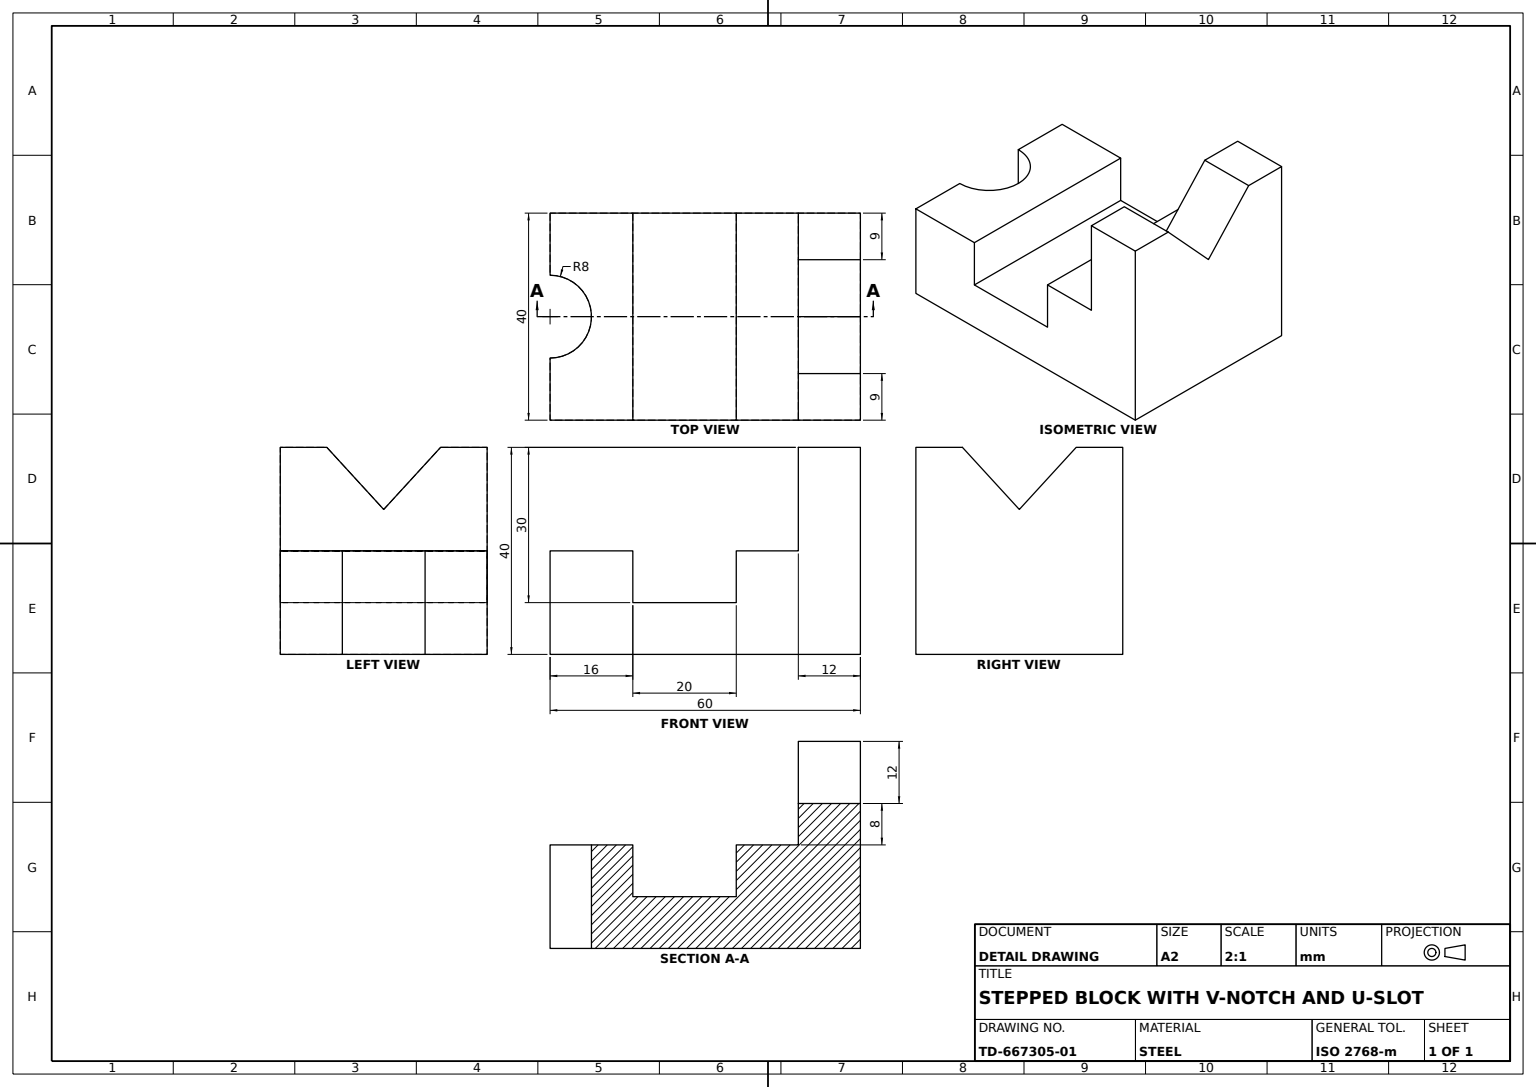
from build123d import *

# Parameters (mm, degrees)
BASE_BODY_DEPTH        = 60
UPRIGHT_PROFILE_W      = 40
UPRIGHT_PROFILE_H      = 20
UPRIGHT_BLOCK_DEPTH    = 12
STEP_CUT_PROFILE_W     = 20
STEP_CUT_PROFILE_H     = 20
STEP_CUT_DEPTH         = 60
HALF_ROUND_NOTCH_DEPTH = 60
CROSS_SLOT_PROFILE_W   = 20
CROSS_SLOT_PROFILE_H   = 10
CROSS_SLOT_DEPTH       = 60
ANGLED_NOTCH_DEPTH     = 60


with BuildPart() as part:
    # Base Profile → Base Body (new body)
    with BuildSketch(Plane.XY):
        Polygon((0, 0), (60, 0), (60, 20), (16, 20), (0, 20), align=None)
    extrude(amount=BASE_BODY_DEPTH)

    # Upright Profile → Upright Block (add)
    with BuildSketch(Plane(origin=(0, 0, 0), x_dir=(-1, 0, 0), z_dir=(0, 0, -1))):
        with Locations((-40, 30)):
            Rectangle(UPRIGHT_PROFILE_W, UPRIGHT_PROFILE_H)
    extrude(amount=-UPRIGHT_BLOCK_DEPTH)

    # Step Cut Profile → Step Cut (cut)
    with BuildSketch(Plane(origin=(0, 0, 0), x_dir=(-1, 0, 0), z_dir=(0, 0, -1))):
        with Locations((-10, 10)):
            Rectangle(STEP_CUT_PROFILE_W, STEP_CUT_PROFILE_H)
    extrude(amount=-STEP_CUT_DEPTH, mode=Mode.SUBTRACT)

    # Half-Round Notch Profile → Half-Round Notch (cut)
    with BuildSketch(Plane(origin=(0, 20, 0), x_dir=(1, 0, 0), z_dir=(0, 1, 0))):
        with BuildLine():
            Line((32, -60), (48, -60))
            ThreePointArc((48, -60), (40, -52), (32, -60))
        make_face()
    extrude(amount=-HALF_ROUND_NOTCH_DEPTH, mode=Mode.SUBTRACT)

    # Cross Slot Profile → Cross Slot (cut)
    with BuildSketch(Plane(origin=(60, 0, 0), x_dir=(0, 0, -1), z_dir=(1, 0, 0))):
        with Locations((-34, 15)):
            Rectangle(CROSS_SLOT_PROFILE_W, CROSS_SLOT_PROFILE_H)
    extrude(amount=-CROSS_SLOT_DEPTH, mode=Mode.SUBTRACT)

    # Angled Notch Profile → Angled Notch (cut)
    with BuildSketch(Plane.XY.offset(12)):
        Polygon((40, 40), (51, 40), (40, 28), (29, 40), align=None)
    extrude(amount=-ANGLED_NOTCH_DEPTH, mode=Mode.SUBTRACT)


solid = part.part
